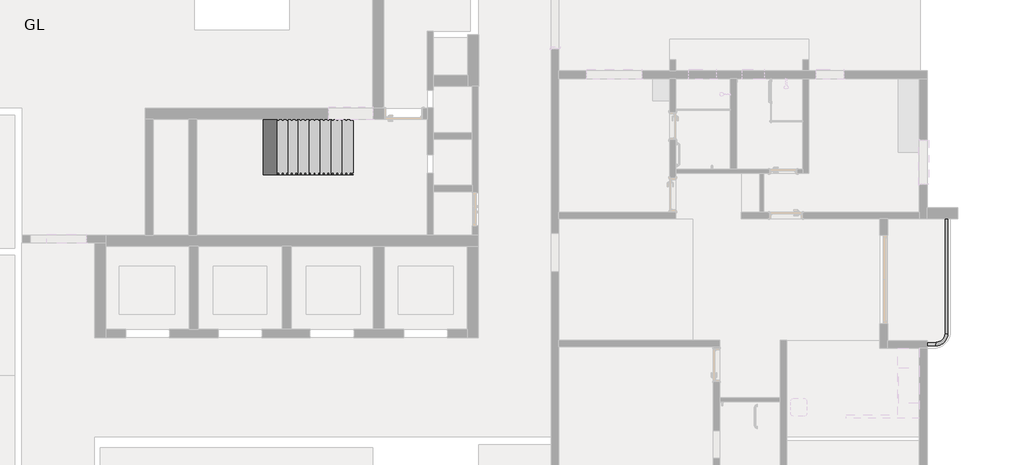
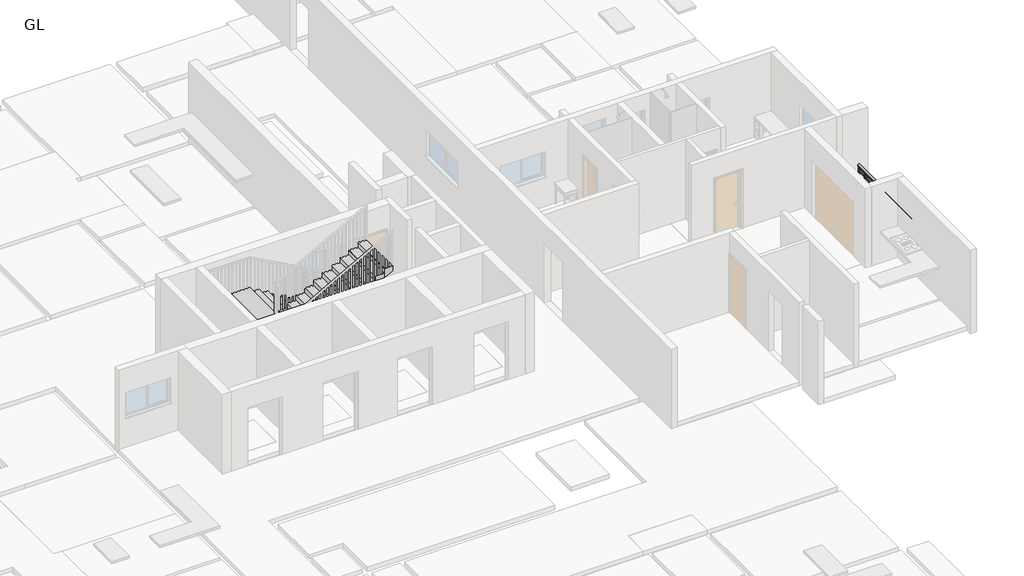
# One storey, part 11 of 14: 1 railing, 1 stair flight.
"""IFC4 building model written with IfcOpenShell, lengths in millimetres."""

from ifc_helpers import new_model, si_unit, point, frame, origin, place, context, project, spatial, polyline, circle_curve, ellipse_curve, trimmed, outline, extrude, faceted_brep, element, save
from ifc_brep_helpers import plane_surface, cylinder_surface, revolved_surface, extruded_surface, advanced_brep

model = new_model("IFC4")

# Units and contexts
model_context = context("Model", 3, world=origin())
ifc_project = project(units=[si_unit("LENGTHUNIT", "METRE", prefix="MILLI")], contexts=[model_context])

# Site, building, storey
site = spatial("IfcSite", under=ifc_project)
building = spatial("IfcBuilding", under=site)
storey = spatial("IfcBuildingStorey", under=building, Name="GL", Elevation=0.0)

# Railing
placement = place(None, origin())
element("IfcRailing", 1, ObjectType="Glass_Panel-Bottom_Fill", at=placement, inside=storey, context=model_context, shape_type="SolidModel", body=[
    advanced_brep(
    [(20240.9477378, 79413.1078957, 1049.9616), (20160.9477378, 79413.1078957, 1049.9616), (20240.9477378, 76242.3017927, 1049.9616), (20160.9477378, 76242.3017927, 1049.9616), (19908.9188628, 75990.2729177, 1049.9616), (19908.9188628, 75910.2729177, 1049.9616), (19668.1569726, 75910.2729177, 1049.9616), (19668.1569726, 75990.2729177, 1049.9616)],
    [
        (0, 1, ellipse_curve(frame((20200.9477378, 79413.1078957, 1049.9616), z_axis=(0.0, 1.0, 0.0), x_axis=(-1.0, 0.0, 0.0)), 40.0, 30.0)),
        (1, 0, ellipse_curve(frame((20200.9477378, 79413.1078957, 1049.9616), z_axis=(0.0, 1.0, 0.0), x_axis=(-1.0, 0.0, 0.0)), 40.0, 30.0)),
        (0, 2),
        (2, 3, ellipse_curve(frame((20200.9477378, 76242.3017927, 1049.9616), z_axis=(0.0, 1.0, 0.0), x_axis=(-1.0, 0.0, 0.0)), 40.0, 30.0)),
        (3, 1),
        (3, 2, ellipse_curve(frame((20200.9477378, 76242.3017927, 1049.9616), z_axis=(0.0, 1.0, 0.0), x_axis=(-1.0, 0.0, 0.0)), 40.0, 30.0)),
        (4, 3, circle_curve(frame((19908.9188628, 76242.3017927, 1049.9616), z_axis=(0.0, 0.0, 1.0), x_axis=(1.0, 0.0, 0.0)), 252.028875)),
        (2, 5, circle_curve(frame((19908.9188628, 76242.3017927, 1049.9616), z_axis=(0.0, 0.0, -1.0), x_axis=(1.0, 0.0, 0.0)), 332.028875)),
        (5, 4, ellipse_curve(frame((19908.9188628, 75950.2729177, 1049.9616), z_axis=(1.0, 0.0, 0.0), x_axis=(0.0, 1.0, 0.0)), 40.0, 30.0)),
        (4, 5, ellipse_curve(frame((19908.9188628, 75950.2729177, 1049.9616), z_axis=(1.0, 0.0, 0.0), x_axis=(0.0, 1.0, 0.0)), 40.0, 30.0)),
        (6, 7, ellipse_curve(frame((19668.1569726, 75950.2729177, 1049.9616), z_axis=(-1.0, 0.0, 0.0), x_axis=(0.0, 1.0, 0.0)), 40.0, 30.0)),
        (7, 6, ellipse_curve(frame((19668.1569726, 75950.2729177, 1049.9616), z_axis=(-1.0, 0.0, 0.0), x_axis=(0.0, 1.0, 0.0)), 40.0, 30.0)),
        (5, 6),
        (7, 4),
    ],
    [
        plane_surface(frame((20200.9477378, 79413.1078957, 1049.9616), z_axis=(0.0, 1.0, 0.0), x_axis=(0.0, 0.0, -1.0))),
        extruded_surface(trimmed(ellipse_curve(frame((20200.9477378, 76242.3017927, 1049.9616), z_axis=(0.0, 1.0, 0.0), x_axis=(-1.0, 0.0, 0.0)), 40.0, 30.0), [point((20240.9477378, 76242.3017927, 1049.9616))], [point((20160.9477378, 76242.3017927, 1049.9616))], True, "CARTESIAN"), (0.0, 3170.8061029999953, 0.0), 3170.8061029999953),
        extruded_surface(trimmed(ellipse_curve(frame((20200.9477378, 76242.3017927, 1049.9616), z_axis=(0.0, 1.0, 0.0), x_axis=(-1.0, 0.0, 0.0)), 40.0, 30.0), [point((20160.9477378, 76242.3017927, 1049.9616))], [point((20240.9477378, 76242.3017927, 1049.9616))], True, "CARTESIAN"), (0.0, 3170.8061029999953, 0.0), 3170.8061029999953),
        revolved_surface(trimmed(ellipse_curve(frame((20200.9477378, 76242.3017927, 1049.9616), z_axis=(0.0, 1.0, 0.0), x_axis=(-1.0, 0.0, 0.0)), 40.0, 30.0), [point((20240.9477378, 76242.3017927, 1049.9616))], [point((20160.9477378, 76242.3017927, 1049.9616))], True, "CARTESIAN"), (19908.9188628, 76242.3017927, 1049.9616), (0.0, 0.0, -1.0)),
        revolved_surface(trimmed(ellipse_curve(frame((20200.9477378, 76242.3017927, 1049.9616), z_axis=(0.0, 1.0, 0.0), x_axis=(-1.0, 0.0, 0.0)), 40.0, 30.0), [point((20160.9477378, 76242.3017927, 1049.9616))], [point((20240.9477378, 76242.3017927, 1049.9616))], True, "CARTESIAN"), (19908.9188628, 76242.3017927, 1049.9616), (0.0, 0.0, -1.0)),
        plane_surface(frame((19668.1569726, 75950.2729177, 1049.9616), z_axis=(-1.0, 0.0, 0.0), x_axis=(0.0, -1.0, 0.0))),
        extruded_surface(trimmed(ellipse_curve(frame((19668.1569726, 75950.2729177, 1049.9616), z_axis=(1.0, 0.0, 0.0), x_axis=(0.0, 1.0, 0.0)), 40.0, 30.0), [point((19668.1569726, 75910.2729177, 1049.9616))], [point((19668.1569726, 75990.2729177, 1049.9616))], True, "CARTESIAN"), (240.76189019999947, 0.0, 0.0), 240.76189019999947),
        extruded_surface(trimmed(ellipse_curve(frame((19668.1569726, 75950.2729177, 1049.9616), z_axis=(1.0, 0.0, 0.0), x_axis=(0.0, 1.0, 0.0)), 40.0, 30.0), [point((19668.1569726, 75990.2729177, 1049.9616))], [point((19668.1569726, 75910.2729177, 1049.9616))], True, "CARTESIAN"), (240.76189019999947, 0.0, 0.0), 240.76189019999947),
    ],
    [
        (0, [[1, 2]]),
        (1, [[-1, 3, 4, 5]]),
        (2, [[-2, -5, 6, -3]]),
        (3, [[7, -4, 8, 9]]),
        (4, [[-8, -6, -7, 10]]),
        (5, [[11, 12]]),
        (6, [[-9, 13, -12, 14]]),
        (7, [[-10, -14, -11, -13]]),
    ],
),
    advanced_brep(
    [(20191.5569726, 79413.1078957, 949.9616), (20211.5569726, 79413.1078957, 949.9616), (20211.5569726, 79413.1078957, 929.9616), (20191.5569726, 79413.1078957, 929.9616), (20191.5569726, 76242.3017927, 949.9616), (20211.5569726, 76242.3017927, 949.9616), (20211.5569726, 76242.3017927, 929.9616), (20191.5569726, 76242.3017927, 929.9616), (19908.9188628, 75939.6636829, 949.9616), (19908.9188628, 75959.6636829, 949.9616), (19908.9188628, 75939.6636829, 929.9616), (19908.9188628, 75959.6636829, 929.9616), (19668.1569726, 75959.6636829, 949.9616), (19668.1569726, 75959.6636829, 929.9616), (19668.1569726, 75939.6636829, 929.9616), (19668.1569726, 75939.6636829, 949.9616)],
    [
        (0, 1),
        (1, 2),
        (2, 3),
        (3, 0),
        (0, 4),
        (4, 5),
        (5, 1),
        (5, 6),
        (6, 2),
        (6, 7),
        (7, 3),
        (7, 4),
        (8, 5, circle_curve(frame((19908.9188628, 76242.3017927, 949.9616), z_axis=(0.0, 0.0, 1.0), x_axis=(1.0, 0.0, 0.0)), 302.6381098)),
        (4, 9, circle_curve(frame((19908.9188628, 76242.3017927, 949.9616), z_axis=(0.0, 0.0, -1.0), x_axis=(1.0, 0.0, 0.0)), 282.6381098)),
        (9, 8),
        (10, 6, circle_curve(frame((19908.9188628, 76242.3017927, 929.9616), z_axis=(0.0, 0.0, 1.0), x_axis=(1.0, 0.0, 0.0)), 302.6381098)),
        (8, 10),
        (11, 7, circle_curve(frame((19908.9188628, 76242.3017927, 929.9616), z_axis=(0.0, 0.0, 1.0), x_axis=(1.0, 0.0, 0.0)), 282.6381098)),
        (10, 11),
        (11, 9),
        (12, 13),
        (13, 14),
        (14, 15),
        (15, 12),
        (9, 12),
        (15, 8),
        (14, 10),
        (13, 11),
    ],
    [
        plane_surface(frame((20201.5569726, 79413.1078957, 949.9616), z_axis=(0.0, 1.0, 0.0), x_axis=(0.0, 0.0, -1.0))),
        plane_surface(frame((20191.5569726, 79413.1078957, 949.9616), z_axis=(0.0, 0.0, 1.0), x_axis=(0.0, -1.0, 0.0))),
        plane_surface(frame((20211.5569726, 79413.1078957, 949.9616), z_axis=(1.0, 0.0, 0.0), x_axis=(0.0, -1.0, 0.0))),
        plane_surface(frame((20211.5569726, 79413.1078957, 929.9616), z_axis=(0.0, 0.0, -1.0), x_axis=(0.0, -1.0, 0.0))),
        plane_surface(frame((20191.5569726, 79413.1078957, 929.9616), z_axis=(-1.0, 0.0, 0.0), x_axis=(0.0, -1.0, 0.0))),
        plane_surface(frame((19908.9188628, 76242.3017927, 949.9616), z_axis=(0.0, 0.0, 1.0), x_axis=(1.0, 0.0, 0.0))),
        cylinder_surface(frame((19908.9188628, 76242.3017927, 949.9616), z_axis=(0.0, 0.0, -1.0), x_axis=(1.0, 0.0, 0.0)), 302.6381098),
        plane_surface(frame((19908.9188628, 76242.3017927, 929.9616), z_axis=(0.0, 0.0, -1.0), x_axis=(1.0, 0.0, 0.0))),
        revolved_surface(polyline([(20191.5569726, 76242.3017927, 929.9616), (20191.5569726, 76242.3017927, 949.9616)]), (19908.9188628, 76242.3017927, 949.9616), (0.0, 0.0, -1.0)),
        plane_surface(frame((19668.1569726, 75949.6636829, 949.9616), z_axis=(-1.0, 0.0, 0.0), x_axis=(0.0, -1.0, 0.0))),
        plane_surface(frame((19908.9188628, 75959.6636829, 949.9616), z_axis=(0.0, 0.0, 1.0), x_axis=(-1.0, 0.0, 0.0))),
        plane_surface(frame((19908.9188628, 75939.6636829, 949.9616), z_axis=(0.0, -1.0, 0.0), x_axis=(-1.0, 0.0, 0.0))),
        plane_surface(frame((19908.9188628, 75939.6636829, 929.9616), z_axis=(0.0, 0.0, -1.0), x_axis=(-1.0, 0.0, 0.0))),
        plane_surface(frame((19908.9188628, 75959.6636829, 929.9616), z_axis=(0.0, 1.0, 0.0), x_axis=(-1.0, 0.0, 0.0))),
    ],
    [
        (0, [[1, 2, 3, 4]]),
        (1, [[-1, 5, 6, 7]]),
        (2, [[-2, -7, 8, 9]]),
        (3, [[-3, -9, 10, 11]]),
        (4, [[-4, -11, 12, -5]]),
        (5, [[13, -6, 14, 15]]),
        (6, [[16, -8, -13, 17]]),
        (7, [[18, -10, -16, 19]]),
        (8, [[-14, -12, -18, 20]]),
        (9, [[21, 22, 23, 24]]),
        (10, [[-15, 25, -24, 26]]),
        (11, [[-17, -26, -23, 27]]),
        (12, [[-19, -27, -22, 28]]),
        (13, [[-20, -28, -21, -25]]),
    ],
),
    advanced_brep(
    [(20191.5569726, 79413.1078957, 849.9616), (20211.5569726, 79413.1078957, 849.9616), (20211.5569726, 79413.1078957, 829.9616), (20191.5569726, 79413.1078957, 829.9616), (20191.5569726, 76242.3017927, 849.9616), (20211.5569726, 76242.3017927, 849.9616), (20211.5569726, 76242.3017927, 829.9616), (20191.5569726, 76242.3017927, 829.9616), (19908.9188628, 75939.6636829, 849.9616), (19908.9188628, 75959.6636829, 849.9616), (19908.9188628, 75939.6636829, 829.9616), (19908.9188628, 75959.6636829, 829.9616), (19668.1569726, 75959.6636829, 849.9616), (19668.1569726, 75959.6636829, 829.9616), (19668.1569726, 75939.6636829, 829.9616), (19668.1569726, 75939.6636829, 849.9616)],
    [
        (0, 1),
        (1, 2),
        (2, 3),
        (3, 0),
        (0, 4),
        (4, 5),
        (5, 1),
        (5, 6),
        (6, 2),
        (6, 7),
        (7, 3),
        (7, 4),
        (8, 5, circle_curve(frame((19908.9188628, 76242.3017927, 849.9616), z_axis=(0.0, 0.0, 1.0), x_axis=(1.0, 0.0, 0.0)), 302.6381098)),
        (4, 9, circle_curve(frame((19908.9188628, 76242.3017927, 849.9616), z_axis=(0.0, 0.0, -1.0), x_axis=(1.0, 0.0, 0.0)), 282.6381098)),
        (9, 8),
        (10, 6, circle_curve(frame((19908.9188628, 76242.3017927, 829.9616), z_axis=(0.0, 0.0, 1.0), x_axis=(1.0, 0.0, 0.0)), 302.6381098)),
        (8, 10),
        (11, 7, circle_curve(frame((19908.9188628, 76242.3017927, 829.9616), z_axis=(0.0, 0.0, 1.0), x_axis=(1.0, 0.0, 0.0)), 282.6381098)),
        (10, 11),
        (11, 9),
        (12, 13),
        (13, 14),
        (14, 15),
        (15, 12),
        (9, 12),
        (15, 8),
        (14, 10),
        (13, 11),
    ],
    [
        plane_surface(frame((20201.5569726, 79413.1078957, 849.9616), z_axis=(0.0, 1.0, 0.0), x_axis=(0.0, 0.0, -1.0))),
        plane_surface(frame((20191.5569726, 79413.1078957, 849.9616), z_axis=(0.0, 0.0, 1.0), x_axis=(0.0, -1.0, 0.0))),
        plane_surface(frame((20211.5569726, 79413.1078957, 849.9616), z_axis=(1.0, 0.0, 0.0), x_axis=(0.0, -1.0, 0.0))),
        plane_surface(frame((20211.5569726, 79413.1078957, 829.9616), z_axis=(0.0, 0.0, -1.0), x_axis=(0.0, -1.0, 0.0))),
        plane_surface(frame((20191.5569726, 79413.1078957, 829.9616), z_axis=(-1.0, 0.0, 0.0), x_axis=(0.0, -1.0, 0.0))),
        plane_surface(frame((19908.9188628, 76242.3017927, 849.9616), z_axis=(0.0, 0.0, 1.0), x_axis=(1.0, 0.0, 0.0))),
        cylinder_surface(frame((19908.9188628, 76242.3017927, 849.9616), z_axis=(0.0, 0.0, -1.0), x_axis=(1.0, 0.0, 0.0)), 302.6381098),
        plane_surface(frame((19908.9188628, 76242.3017927, 829.9616), z_axis=(0.0, 0.0, -1.0), x_axis=(1.0, 0.0, 0.0))),
        revolved_surface(polyline([(20191.5569726, 76242.3017927, 829.9616), (20191.5569726, 76242.3017927, 849.9616)]), (19908.9188628, 76242.3017927, 849.9616), (0.0, 0.0, -1.0)),
        plane_surface(frame((19668.1569726, 75949.6636829, 849.9616), z_axis=(-1.0, 0.0, 0.0), x_axis=(0.0, -1.0, 0.0))),
        plane_surface(frame((19908.9188628, 75959.6636829, 849.9616), z_axis=(0.0, 0.0, 1.0), x_axis=(-1.0, 0.0, 0.0))),
        plane_surface(frame((19908.9188628, 75939.6636829, 849.9616), z_axis=(0.0, -1.0, 0.0), x_axis=(-1.0, 0.0, 0.0))),
        plane_surface(frame((19908.9188628, 75939.6636829, 829.9616), z_axis=(0.0, 0.0, -1.0), x_axis=(-1.0, 0.0, 0.0))),
        plane_surface(frame((19908.9188628, 75959.6636829, 829.9616), z_axis=(0.0, 1.0, 0.0), x_axis=(-1.0, 0.0, 0.0))),
    ],
    [
        (0, [[1, 2, 3, 4]]),
        (1, [[-1, 5, 6, 7]]),
        (2, [[-2, -7, 8, 9]]),
        (3, [[-3, -9, 10, 11]]),
        (4, [[-4, -11, 12, -5]]),
        (5, [[13, -6, 14, 15]]),
        (6, [[16, -8, -13, 17]]),
        (7, [[18, -10, -16, 19]]),
        (8, [[-14, -12, -18, 20]]),
        (9, [[21, 22, 23, 24]]),
        (10, [[-15, 25, -24, 26]]),
        (11, [[-17, -26, -23, 27]]),
        (12, [[-19, -27, -22, 28]]),
        (13, [[-20, -28, -21, -25]]),
    ],
),
    extrude(outline(polyline([(20226.5569726, 76633.7048442), (20226.5569726, 76621.7048442), (20176.5569726, 76621.7048442), (20176.5569726, 76633.7048442), (20226.5569726, 76633.7048442)])), frame((0.0, 0.0, 149.9616), z_axis=(0.0, 0.0, 1.0), x_axis=(1.0, 0.0, 0.0)), (0.0, 0.0, 1.0), 870.0),
    extrude(outline(polyline([(20199.8321625, 77427.7048442), (20199.8321625, 76627.7048442), (20194.8321625, 76627.7048442), (20194.8321625, 77427.7048442), (20199.8321625, 77427.7048442)])), frame((0.0, 0.0, 249.9616), z_axis=(0.0, 0.0, 1.0), x_axis=(1.0, 0.0, 0.0)), (0.0, 0.0, 1.0), 580.0),
    extrude(outline(polyline([(20226.5569726, 77433.7048442), (20226.5569726, 77421.7048442), (20176.5569726, 77421.7048442), (20176.5569726, 77433.7048442), (20226.5569726, 77433.7048442)])), frame((0.0, 0.0, 149.9616), z_axis=(0.0, 0.0, 1.0), x_axis=(1.0, 0.0, 0.0)), (0.0, 0.0, 1.0), 870.0),
    extrude(outline(polyline([(20199.8321625, 78227.7048442), (20199.8321625, 77427.7048442), (20194.8321625, 77427.7048442), (20194.8321625, 78227.7048442), (20199.8321625, 78227.7048442)])), frame((0.0, 0.0, 249.9616), z_axis=(0.0, 0.0, 1.0), x_axis=(1.0, 0.0, 0.0)), (0.0, 0.0, 1.0), 580.0),
    extrude(outline(polyline([(20226.5569726, 78233.7048442), (20226.5569726, 78221.7048442), (20176.5569726, 78221.7048442), (20176.5569726, 78233.7048442), (20226.5569726, 78233.7048442)])), frame((0.0, 0.0, 149.9616), z_axis=(0.0, 0.0, 1.0), x_axis=(1.0, 0.0, 0.0)), (0.0, 0.0, 1.0), 870.0),
    extrude(outline(polyline([(20199.8321625, 79027.7048442), (20199.8321625, 78227.7048442), (20194.8321625, 78227.7048442), (20194.8321625, 79027.7048442), (20199.8321625, 79027.7048442)])), frame((0.0, 0.0, 249.9616), z_axis=(0.0, 0.0, 1.0), x_axis=(1.0, 0.0, 0.0)), (0.0, 0.0, 1.0), 580.0),
    extrude(outline(polyline([(20226.5569726, 79033.7048442), (20226.5569726, 79021.7048442), (20176.5569726, 79021.7048442), (20176.5569726, 79033.7048442), (20226.5569726, 79033.7048442)])), frame((0.0, 0.0, 149.9616), z_axis=(0.0, 0.0, 1.0), x_axis=(1.0, 0.0, 0.0)), (0.0, 0.0, 1.0), 870.0),
    extrude(outline(polyline([(19914.9188628, 75924.6636829), (19902.9188628, 75924.6636829), (19902.9188628, 75974.6636829), (19914.9188628, 75974.6636829), (19914.9188628, 75924.6636829)])), frame((0.0, 0.0, 149.9616), z_axis=(0.0, 0.0, 1.0), x_axis=(1.0, 0.0, 0.0)), (0.0, 0.0, 1.0), 870.0),
    extrude(outline(polyline([(20226.5569726, 76248.3017927), (20226.5569726, 76236.3017927), (20176.5569726, 76236.3017927), (20176.5569726, 76248.3017927), (20226.5569726, 76248.3017927)])), frame((0.0, 0.0, 149.9616), z_axis=(0.0, 0.0, 1.0), x_axis=(1.0, 0.0, 0.0)), (0.0, 0.0, 1.0), 870.0),
    extrude(outline(polyline([(19676.1569726, 75924.6636829), (19664.1569726, 75924.6636829), (19664.1569726, 75974.6636829), (19676.1569726, 75974.6636829), (19676.1569726, 75924.6636829)])), frame((0.0, 0.0, 149.9616), z_axis=(0.0, 0.0, 1.0), x_axis=(1.0, 0.0, 0.0)), (0.0, 0.0, 1.0), 870.0),
    extrude(outline(polyline([(20226.5569726, 79417.1078957), (20226.5569726, 79405.1078957), (20176.5569726, 79405.1078957), (20176.5569726, 79417.1078957), (20226.5569726, 79417.1078957)])), frame((0.0, 0.0, 149.9616), z_axis=(0.0, 0.0, 1.0), x_axis=(1.0, 0.0, 0.0)), (0.0, 0.0, 1.0), 870.0),
])

# Stair flight
element("IfcStairFlight", 2, ObjectType="1mm_Tread-150mm_Depth", at=placement, inside=storey, context=model_context, shape_type="SolidModel", body=[
    faceted_brep([(3526.0691495, 80618.1615983, 165.6666667), (3830.8691495, 80618.1615983, 165.6666667), (3830.8691495, 82157.7073985, 165.6666667), (3526.0691495, 82157.7073985, 165.6666667), (3526.0691495, 80618.1615983, 0.0), (3830.8691495, 80618.1615983, 0.0), (3830.8691495, 82157.7073985, 0.0), (3526.0691495, 82157.7073985, 0.0), (3221.2691495, 80618.1615983, 332.3333333), (3526.0691495, 80618.1615983, 332.3333333), (3526.0691495, 82157.7073985, 332.3333333), (3221.2691495, 82157.7073985, 332.3333333), (3221.2691495, 80618.1615983, 164.8133213), (3519.191203, 80618.1615983, 0.0), (3519.191203, 82157.7073985, 0.0), (3221.2691495, 82157.7073985, 164.8133213), (2916.4691495, 80618.1615983, 499.0), (3221.2691495, 80618.1615983, 499.0), (3221.2691495, 82157.7073985, 499.0), (2916.4691495, 82157.7073985, 499.0), (2916.4691495, 80618.1615983, 333.4315883), (2916.4691495, 82157.7073985, 333.4315883), (2611.6691495, 80618.1615983, 665.6666667), (2916.4691495, 80618.1615983, 665.6666667), (2916.4691495, 82157.7073985, 665.6666667), (2611.6691495, 82157.7073985, 665.6666667), (2611.6691495, 80618.1615983, 502.0498553), (2611.6691495, 82157.7073985, 502.0498553), (2306.8691495, 80618.1615983, 832.3333333), (2611.6691495, 80618.1615983, 832.3333333), (2611.6691495, 82157.7073985, 832.3333333), (2306.8691495, 82157.7073985, 832.3333333), (2306.8691495, 80618.1615983, 670.6681223), (2306.8691495, 82157.7073985, 670.6681223), (2027.4691495, 80618.1615983, 999.0), (2306.8691495, 80618.1615983, 999.0), (2306.8691495, 82157.7073985, 999.0), (2027.4691495, 82157.7073985, 999.0), (2027.4691495, 80618.1615983, 825.234867), (2027.4691495, 82157.7073985, 825.234867), (1722.6691495, 80618.1615983, 1165.6666667), (2027.4691495, 80618.1615983, 1165.6666667), (2027.4691495, 82157.7073985, 1165.6666667), (1722.6691495, 82157.7073985, 1165.6666667), (1722.6691495, 80618.1615983, 993.853134), (1722.6691495, 82157.7073985, 993.853134), (1424.2191495, 80618.1615983, 1332.3333333), (1722.6691495, 80618.1615983, 1332.3333333), (1722.6691495, 82157.7073985, 1332.3333333), (1424.2191495, 82157.7073985, 1332.3333333), (1424.2191495, 80618.1615983, 1158.9585204), (1424.2191495, 82157.7073985, 1158.9585204), (1119.4191495, 80618.1615983, 1499.0), (1424.2191495, 80618.1615983, 1499.0), (1424.2191495, 82157.7073985, 1499.0), (1119.4191495, 82157.7073985, 1499.0), (1119.4191495, 80618.1615983, 1515.6666667), (779.4216141, 80618.1615983, 1515.6666667), (1119.4191495, 82157.7073985, 1327.5767874), (1119.4191495, 80493.8950959, 1665.6666667), (1119.4191495, 80618.1615983, 1665.6666667), (1119.4191495, 82157.7073985, 1665.6666667), (779.4216141, 82157.7073985, 1665.6666667), (-478.6271613, 82157.7073985, 1665.6666667), (-478.6271613, 78948.3487724, 1665.6666667), (1119.4191495, 78948.3487724, 1665.6666667), (1119.4191495, 80493.8950959, 1515.6666667), (779.4216141, 82157.7073985, 1515.6666667), (-478.6271613, 82157.7073985, 1515.6666667), (-478.6271613, 78948.3487724, 1515.6666667), (1119.4191495, 78948.3487724, 1515.6666667), (1119.4191495, 80493.8950959, 1832.3333333), (1119.4191495, 78948.3487724, 1832.3333333), (1158.1444628, 78948.3487724, 1832.3333333), (1424.2191495, 78948.3487724, 1832.3333333), (1424.2191495, 80493.8950959, 1832.3333333), (1158.1444628, 80493.8950959, 1832.3333333), (1424.2191495, 80493.8950959, 1662.861721), (1158.1444628, 80493.8950959, 1515.6666667), (1158.1444628, 78948.3487724, 1515.6666667), (1424.2191495, 78948.3487724, 1662.861721), (1722.6691495, 80493.8950959, 1999.0), (1424.2191495, 80493.8950959, 1999.0), (1424.2191495, 78948.3487724, 1999.0), (1722.6691495, 78948.3487724, 1999.0), (1722.6691495, 80493.8950959, 1827.9671074), (1722.6691495, 78948.3487724, 1827.9671074), (2021.1191495, 80493.8950959, 2165.6666667), (1722.6691495, 80493.8950959, 2165.6666667), (1722.6691495, 78948.3487724, 2165.6666667), (2021.1191495, 78948.3487724, 2165.6666667), (2021.1191495, 80493.8950959, 1993.0724939), (2021.1191495, 78948.3487724, 1993.0724939), (2319.5691495, 80493.8950959, 2332.3333333), (2021.1191495, 80493.8950959, 2332.3333333), (2021.1191495, 78948.3487724, 2332.3333333), (2319.5691495, 78948.3487724, 2332.3333333), (2319.5691495, 80493.8950959, 2158.1778803), (2319.5691495, 78948.3487724, 2158.1778803), (2618.0191495, 80493.8950959, 2499.0), (2319.5691495, 80493.8950959, 2499.0), (2319.5691495, 78948.3487724, 2499.0), (2618.0191495, 78948.3487724, 2499.0), (2618.0191495, 80493.8950959, 2323.2832667), (2618.0191495, 78948.3487724, 2323.2832667), (2929.1691495, 80493.8950959, 2665.6666667), (2618.0191495, 80493.8950959, 2665.6666667), (2618.0191495, 78948.3487724, 2665.6666667), (2929.1691495, 78948.3487724, 2665.6666667), (2929.1691495, 80493.8950959, 2495.4144142), (2929.1691495, 78948.3487724, 2495.4144142), (3227.6191495, 80493.8950959, 2832.3333333), (2929.1691495, 80493.8950959, 2832.3333333), (2929.1691495, 78948.3487724, 2832.3333333), (3227.6191495, 78948.3487724, 2832.3333333), (3227.6191495, 80493.8950959, 2660.5198007), (3227.6191495, 78948.3487724, 2660.5198007), (3526.0691495, 80493.8950959, 2999.0), (3227.6191495, 80493.8950959, 2999.0), (3227.6191495, 78948.3487724, 2999.0), (3526.0691495, 78948.3487724, 2999.0), (3526.0691495, 80493.8950959, 2825.6251871), (3526.0691495, 78948.3487724, 2825.6251871), (3830.8691495, 80493.8950959, 3165.6666667), (3526.0691495, 80493.8950959, 3165.6666667), (3526.0691495, 78948.3487724, 3165.6666667), (3830.8691495, 78948.3487724, 3165.6666667), (3830.8691495, 80493.8950959, 2994.243454), (3830.8691495, 78948.3487724, 2994.243454), (4118.7728387, 80493.8950959, 3332.3333333), (3830.8691495, 80493.8950959, 3332.3333333), (3830.8691495, 78948.3487724, 3332.3333333), (4118.7728387, 78948.3487724, 3332.3333333), (4118.7728387, 80493.8950959, 3153.5145207), (4118.7728387, 78948.3487724, 3153.5145207)], [[[0, 1, 2, 3]], [[1, 0, 4, 5]], [[2, 1, 5, 6]], [[3, 2, 6, 7]], [[8, 9, 10, 11]], [[4, 0, 9, 8, 12, 13]], [[0, 3, 10, 9]], [[3, 7, 14, 15, 11, 10]], [[16, 17, 18, 19]], [[17, 16, 20, 12, 8]], [[8, 11, 18, 17]], [[19, 18, 11, 15, 21]], [[22, 23, 24, 25]], [[23, 22, 26, 20, 16]], [[16, 19, 24, 23]], [[25, 24, 19, 21, 27]], [[28, 29, 30, 31]], [[29, 28, 32, 26, 22]], [[22, 25, 30, 29]], [[31, 30, 25, 27, 33]], [[34, 35, 36, 37]], [[35, 34, 38, 32, 28]], [[28, 31, 36, 35]], [[37, 36, 31, 33, 39]], [[40, 41, 42, 43]], [[41, 40, 44, 38, 34]], [[34, 37, 42, 41]], [[43, 42, 37, 39, 45]], [[46, 47, 48, 49]], [[47, 46, 50, 44, 40]], [[40, 43, 48, 47]], [[49, 48, 43, 45, 51]], [[52, 53, 54, 55]], [[53, 52, 56, 57, 50, 46]], [[46, 49, 54, 53]], [[55, 54, 49, 51, 58]], [[59, 60, 61, 62, 63, 64, 65]], [[60, 59, 66, 56]], [[52, 55, 61, 60, 56]], [[61, 55, 58, 67, 68, 63, 62]], [[64, 63, 68, 69]], [[65, 64, 69, 70]], [[71, 72, 73, 74, 75, 76]], [[59, 71, 76, 75, 77, 78, 66]], [[59, 65, 72, 71]], [[72, 65, 70, 79, 80, 74, 73]], [[81, 82, 83, 84]], [[82, 81, 85, 77, 75]], [[75, 74, 83, 82]], [[84, 83, 74, 80, 86]], [[87, 88, 89, 90]], [[88, 87, 91, 85, 81]], [[81, 84, 89, 88]], [[90, 89, 84, 86, 92]], [[93, 94, 95, 96]], [[94, 93, 97, 91, 87]], [[87, 90, 95, 94]], [[96, 95, 90, 92, 98]], [[99, 100, 101, 102]], [[100, 99, 103, 97, 93]], [[93, 96, 101, 100]], [[102, 101, 96, 98, 104]], [[105, 106, 107, 108]], [[106, 105, 109, 103, 99]], [[99, 102, 107, 106]], [[108, 107, 102, 104, 110]], [[111, 112, 113, 114]], [[112, 111, 115, 109, 105]], [[105, 108, 113, 112]], [[114, 113, 108, 110, 116]], [[117, 118, 119, 120]], [[118, 117, 121, 115, 111]], [[111, 114, 119, 118]], [[120, 119, 114, 116, 122]], [[123, 124, 125, 126]], [[124, 123, 127, 121, 117]], [[117, 120, 125, 124]], [[126, 125, 120, 122, 128]], [[129, 130, 131, 132]], [[130, 129, 133, 127, 123]], [[123, 126, 131, 130]], [[132, 131, 126, 128, 134]], [[129, 132, 134, 133]], [[5, 4, 13, 14, 7, 6]], [[50, 57, 67, 58, 51, 45, 39, 33, 27, 21, 15, 14, 13, 12, 20, 26, 32, 38, 44]], [[67, 57, 56, 66, 78, 79, 70, 69, 68]], [[79, 78, 77, 85, 91, 97, 103, 109, 115, 121, 127, 133, 134, 128, 122, 116, 110, 104, 98, 92, 86, 80]]]),
    extrude(outline(polyline([(3526.0691495, 80618.1615983), (3526.0691495, 82157.7073985), (3830.8691495, 82157.7073985), (3830.8691495, 80618.1615983), (3526.0691495, 80618.1615983)])), frame((0.0, 0.0, 165.6666667), z_axis=(0.0, 0.0, 1.0), x_axis=(1.0, 0.0, 0.0)), (0.0, 0.0, 1.0), 1.0),
    extrude(outline(polyline([(3221.2691495, 80618.1615983), (3221.2691495, 82157.7073985), (3526.0691495, 82157.7073985), (3526.0691495, 80618.1615983), (3221.2691495, 80618.1615983)])), frame((0.0, 0.0, 332.3333333), z_axis=(0.0, 0.0, 1.0), x_axis=(1.0, 0.0, 0.0)), (0.0, 0.0, 1.0), 1.0),
    extrude(outline(polyline([(2916.4691495, 80618.1615983), (2916.4691495, 82157.7073985), (3221.2691495, 82157.7073985), (3221.2691495, 80618.1615983), (2916.4691495, 80618.1615983)])), frame((0.0, 0.0, 499.0), z_axis=(0.0, 0.0, 1.0), x_axis=(1.0, 0.0, 0.0)), (0.0, 0.0, 1.0), 1.0),
    extrude(outline(polyline([(2611.6691495, 80618.1615983), (2611.6691495, 82157.7073985), (2916.4691495, 82157.7073985), (2916.4691495, 80618.1615983), (2611.6691495, 80618.1615983)])), frame((0.0, 0.0, 665.6666667), z_axis=(0.0, 0.0, 1.0), x_axis=(1.0, 0.0, 0.0)), (0.0, 0.0, 1.0), 1.0),
    extrude(outline(polyline([(2306.8691495, 80618.1615983), (2306.8691495, 82157.7073985), (2611.6691495, 82157.7073985), (2611.6691495, 80618.1615983), (2306.8691495, 80618.1615983)])), frame((0.0, 0.0, 832.3333333), z_axis=(0.0, 0.0, 1.0), x_axis=(1.0, 0.0, 0.0)), (0.0, 0.0, 1.0), 1.0),
    extrude(outline(polyline([(2027.4691495, 80618.1615983), (2027.4691495, 82157.7073985), (2306.8691495, 82157.7073985), (2306.8691495, 80618.1615983), (2027.4691495, 80618.1615983)])), frame((0.0, 0.0, 999.0), z_axis=(0.0, 0.0, 1.0), x_axis=(1.0, 0.0, 0.0)), (0.0, 0.0, 1.0), 1.0),
    extrude(outline(polyline([(1722.6691495, 80618.1615983), (1722.6691495, 82157.7073985), (2027.4691495, 82157.7073985), (2027.4691495, 80618.1615983), (1722.6691495, 80618.1615983)])), frame((0.0, 0.0, 1165.6666667), z_axis=(0.0, 0.0, 1.0), x_axis=(1.0, 0.0, 0.0)), (0.0, 0.0, 1.0), 1.0),
    extrude(outline(polyline([(1424.2191495, 80618.1615983), (1424.2191495, 82157.7073985), (1722.6691495, 82157.7073985), (1722.6691495, 80618.1615983), (1424.2191495, 80618.1615983)])), frame((0.0, 0.0, 1332.3333333), z_axis=(0.0, 0.0, 1.0), x_axis=(1.0, 0.0, 0.0)), (0.0, 0.0, 1.0), 1.0),
    extrude(outline(polyline([(1119.4191495, 80618.1615983), (1119.4191495, 82157.7073985), (1424.2191495, 82157.7073985), (1424.2191495, 80618.1615983), (1119.4191495, 80618.1615983)])), frame((0.0, 0.0, 1499.0), z_axis=(0.0, 0.0, 1.0), x_axis=(1.0, 0.0, 0.0)), (0.0, 0.0, 1.0), 1.0),
    extrude(outline(polyline([(1119.4191495, 80493.8950959), (1119.4191495, 78948.3487724), (-478.6271613, 78948.3487724), (-478.6271613, 82157.7073985), (1119.4191495, 82157.7073985), (1119.4191495, 80618.1615983), (1119.4191495, 80493.8950959)])), frame((0.0, 0.0, 1665.6666667), z_axis=(0.0, 0.0, 1.0), x_axis=(1.0, 0.0, 0.0)), (0.0, 0.0, 1.0), 1.0),
    extrude(outline(polyline([(1424.2191495, 80493.8950959), (1424.2191495, 78948.3487724), (1119.4191495, 78948.3487724), (1119.4191495, 80493.8950959), (1424.2191495, 80493.8950959)])), frame((0.0, 0.0, 1832.3333333), z_axis=(0.0, 0.0, 1.0), x_axis=(1.0, 0.0, 0.0)), (0.0, 0.0, 1.0), 1.0),
    extrude(outline(polyline([(1722.6691495, 80493.8950959), (1722.6691495, 78948.3487724), (1424.2191495, 78948.3487724), (1424.2191495, 80493.8950959), (1722.6691495, 80493.8950959)])), frame((0.0, 0.0, 1999.0), z_axis=(0.0, 0.0, 1.0), x_axis=(1.0, 0.0, 0.0)), (0.0, 0.0, 1.0), 1.0),
    extrude(outline(polyline([(2021.1191495, 80493.8950959), (2021.1191495, 78948.3487724), (1722.6691495, 78948.3487724), (1722.6691495, 80493.8950959), (2021.1191495, 80493.8950959)])), frame((0.0, 0.0, 2165.6666667), z_axis=(0.0, 0.0, 1.0), x_axis=(1.0, 0.0, 0.0)), (0.0, 0.0, 1.0), 1.0),
    extrude(outline(polyline([(2319.5691495, 80493.8950959), (2319.5691495, 78948.3487724), (2021.1191495, 78948.3487724), (2021.1191495, 80493.8950959), (2319.5691495, 80493.8950959)])), frame((0.0, 0.0, 2332.3333333), z_axis=(0.0, 0.0, 1.0), x_axis=(1.0, 0.0, 0.0)), (0.0, 0.0, 1.0), 1.0),
    extrude(outline(polyline([(2618.0191495, 80493.8950959), (2618.0191495, 78948.3487724), (2319.5691495, 78948.3487724), (2319.5691495, 80493.8950959), (2618.0191495, 80493.8950959)])), frame((0.0, 0.0, 2499.0), z_axis=(0.0, 0.0, 1.0), x_axis=(1.0, 0.0, 0.0)), (0.0, 0.0, 1.0), 1.0),
    extrude(outline(polyline([(2929.1691495, 80493.8950959), (2929.1691495, 78948.3487724), (2618.0191495, 78948.3487724), (2618.0191495, 80493.8950959), (2929.1691495, 80493.8950959)])), frame((0.0, 0.0, 2665.6666667), z_axis=(0.0, 0.0, 1.0), x_axis=(1.0, 0.0, 0.0)), (0.0, 0.0, 1.0), 1.0),
    extrude(outline(polyline([(3227.6191495, 80493.8950959), (3227.6191495, 78948.3487724), (2929.1691495, 78948.3487724), (2929.1691495, 80493.8950959), (3227.6191495, 80493.8950959)])), frame((0.0, 0.0, 2832.3333333), z_axis=(0.0, 0.0, 1.0), x_axis=(1.0, 0.0, 0.0)), (0.0, 0.0, 1.0), 1.0),
    extrude(outline(polyline([(3526.0691495, 80493.8950959), (3526.0691495, 78948.3487724), (3227.6191495, 78948.3487724), (3227.6191495, 80493.8950959), (3526.0691495, 80493.8950959)])), frame((0.0, 0.0, 2999.0), z_axis=(0.0, 0.0, 1.0), x_axis=(1.0, 0.0, 0.0)), (0.0, 0.0, 1.0), 1.0),
    extrude(outline(polyline([(3830.8691495, 80493.8950959), (3830.8691495, 78948.3487724), (3526.0691495, 78948.3487724), (3526.0691495, 80493.8950959), (3830.8691495, 80493.8950959)])), frame((0.0, 0.0, 3165.6666667), z_axis=(0.0, 0.0, 1.0), x_axis=(1.0, 0.0, 0.0)), (0.0, 0.0, 1.0), 1.0),
    extrude(outline(polyline([(4118.7728387, 80493.8950959), (4118.7728387, 78948.3487724), (3830.8691495, 78948.3487724), (3830.8691495, 80493.8950959), (4118.7728387, 80493.8950959)])), frame((0.0, 0.0, 3332.3333333), z_axis=(0.0, 0.0, 1.0), x_axis=(1.0, 0.0, 0.0)), (0.0, 0.0, 1.0), 1.0),
])

save(model, "model.ifc")

# Revit data of these elements
# Type "Glass_Panel-Bottom_Fill"
#   built-in parameter 1008612 = 0.019685 (stored number, unit not read)
#   built-in parameter 1008611 = 0.019685 (stored number, unit not read)
#   built-in parameter 1008609 = 0.902231 (stored number, unit not read)
#   built-in parameter 1008604 = 0.19685 (stored number, unit not read)
#   built-in parameter 1008603 = 0.164042 (stored number, unit not read)
#   Railing Height = 2.952756 ft
#   built-in parameter 1008630 = 2
#   built-in parameter 1008610 = 2
# Element 1 (IfcRailing, "Glass_Panel-Bottom_Fill")
#   built-in parameter 1008621 = 0.492 (stored number, unit not read)
#   Phase Created = New Construction
#   Materials on its faces: "Metal - Stainless Steel,Polished", "Glass"
# Element 2 (IfcStairFlight, "1mm_Tread-150mm_Depth")
#   Phase Created = New Construction
#   Materials on its faces: "STAIRCASE"
# Materials
#   "Metal - Stainless Steel,Polished": class "Metal", colour RGB 236 239 239, transparency 0, Cost = 0
#   "Glass": class "Glass", colour RGB 0 128 192, transparency 0.9, Description = "Soda Lime Glass", Cost = 0
#   "STAIRCASE": class "Generic", colour RGB 120 120 120, transparency 0, Cost = 0
